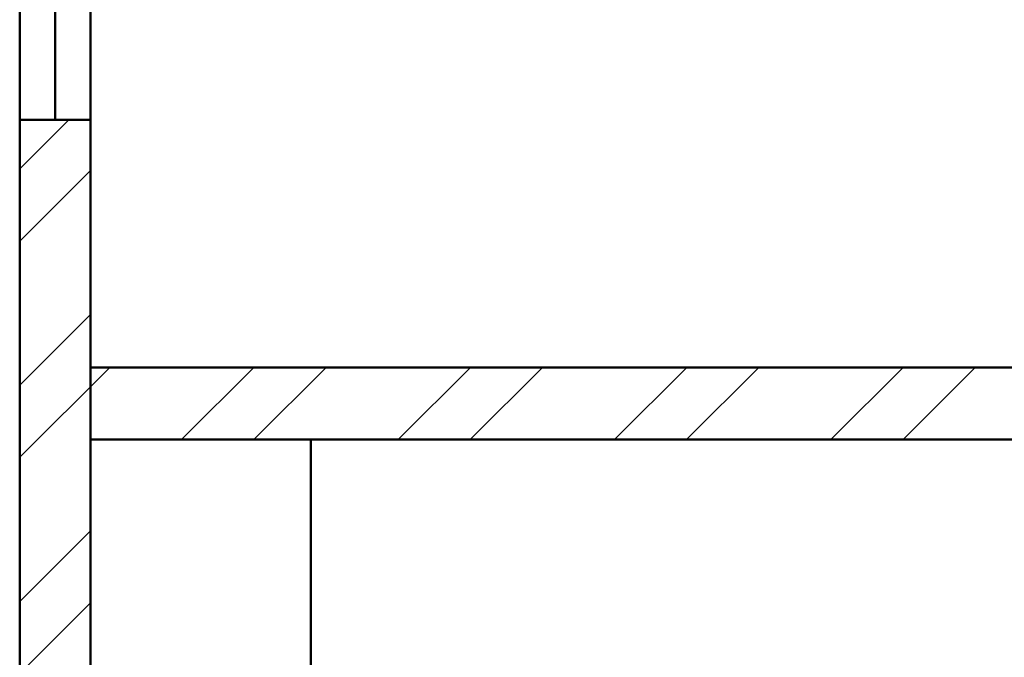
# Model space of a CAD drawing. Units: inches. Extents: x 1901 to 2863, y 888 to 2433.
# Tile 7 of 91: x 2025 to 2086, y 1510 to 1549. Entities that reach past the tile are written whole.
import ezdxf

# ---------------------------------------------------------------- set-up
doc = ezdxf.new("R2010")
doc.units = ezdxf.units.IN
doc.layers.add('A-WALL', color=7, linetype='Continuous', lineweight=50)
doc.layers.add('A-WALL-PATT', color=8, linetype='Continuous', lineweight=13)

msp = doc.modelspace()

# ---------------------------------------------------------------- hatches: boundary and pattern name
at = {"layer": 'A-WALL-PATT'}
h = msp.add_hatch(dxfattribs=at)
h.set_pattern_fill('ANSI32', color=256)
h.paths.add_polyline_path([(2182.933, 1716.634), (2024.926, 1716.634), (2024.926, 1681.702), (2029.326, 1681.702), (2029.326, 1712.134), (2154.326, 1712.134), (2154.326, 1580.134), (2148.524, 1580.134), (2148.524, 1577.884), (2148.524, 1575.634), (2194.93, 1575.634), (2194.93, 1580.134), (2158.826, 1580.134), (2158.826, 1712.134), (2182.933, 1712.134)])
h.paths.add_polyline_path([(2301.069, 1716.634), (2242.933, 1716.634), (2242.933, 1712.134), (2283.826, 1712.134), (2283.826, 1685.535), (2288.326, 1685.535), (2288.326, 1712.134), (2301.069, 1712.134)])
h.paths.add_polyline_path([(2288.326, 1600.411), (2286.076, 1600.411), (2283.826, 1600.411), (2283.826, 1580.134), (2270.601, 1580.134), (2270.601, 1575.634), (2288.326, 1575.634)])
h.paths.add_polyline_path([(2295.926, 1953.634), (2271.447, 1953.634), (2271.447, 1949.134), (2291.426, 1949.134), (2291.426, 1941.244), (2295.926, 1941.244)])
h.paths.add_polyline_path([(2098.376, 1244.134), (2082.326, 1244.134), (2082.326, 1302.134), (2086.523, 1302.134), (2086.523, 1306.634), (2067.456, 1306.634), (2067.456, 1302.134), (2077.826, 1302.134), (2077.826, 1239.634), (2098.376, 1239.634), (2098.376, 1241.884)])
h.paths.add_polyline_path([(2217.308, 1306.634), (2158.826, 1306.634), (2158.826, 1451.634), (2162.716, 1451.634), (2162.716, 1453.884), (2162.716, 1456.134), (2154.326, 1456.134), (2154.326, 1443.134), (2151.91, 1443.134), (2151.91, 1438.634), (2154.326, 1438.634), (2154.326, 1306.634), (2109.307, 1306.634), (2109.307, 1304.384), (2109.307, 1302.134), (2154.326, 1302.134), (2154.326, 1244.134), (2122.376, 1244.134), (2122.376, 1239.634), (2154.326, 1239.634), (2154.326, 1223.634), (2163.326, 1223.634), (2181.008, 1223.634), (2181.008, 1225.884), (2181.008, 1228.134), (2163.326, 1228.134), (2163.326, 1258.222), (2158.826, 1258.222), (2158.826, 1302.134), (2217.308, 1302.134)])
h.paths.add_polyline_path([(2259.991, 1306.634), (2238.299, 1306.634), (2238.299, 1304.384), (2238.299, 1302.134), (2242.826, 1302.134), (2242.826, 1228.134), (2205.008, 1228.134), (2205.008, 1223.634), (2247.326, 1223.634), (2247.326, 1302.134), (2259.991, 1302.134), (2259.991, 1304.384)])
h.paths.add_polyline_path([(2343.426, 1361.697), (2338.926, 1361.697), (2338.926, 1306.634), (2322.38, 1306.634), (2322.38, 1302.134), (2343.426, 1302.134)])
h.paths.add_polyline_path([(2343.426, 1470.397), (2338.926, 1470.397), (2338.926, 1456.134), (2193.726, 1456.134), (2193.726, 1453.884), (2193.726, 1451.634), (2338.926, 1451.634), (2338.926, 1421.697), (2343.426, 1421.697)])
h.paths.add_polyline_path([(2343.426, 1545.507), (2338.926, 1545.507), (2338.926, 1530.397), (2343.426, 1530.397)])
h.paths.add_polyline_path([(2029.326, 1466.83), (2024.926, 1466.83), (2024.926, 1409.825), (2029.326, 1409.825)])
h.paths.add_polyline_path([(2122.843, 1440.884), (2122.843, 1443.134), (2121.826, 1443.134), (2121.826, 1498.183), (2119.576, 1498.183), (2117.326, 1498.183), (2117.326, 1443.134), (2029.326, 1443.134), (2029.326, 1438.634), (2122.843, 1438.634)])
h.paths.add_polyline_path([(2029.326, 1543.053), (2024.926, 1543.053), (2024.926, 1502.83), (2029.326, 1502.83)])
h.paths.add_polyline_path([(2029.326, 1621.702), (2024.926, 1621.702), (2024.926, 1567.053), (2027.126, 1567.053), (2029.326, 1567.053), (2029.326, 1575.634), (2109.326, 1575.634), (2109.326, 1554.715), (2113.826, 1554.715), (2113.826, 1575.634), (2115.805, 1575.634), (2115.805, 1577.884), (2115.805, 1580.134), (2029.326, 1580.134)])
h.paths.add_polyline_path([(2121.826, 1527.634), (2117.326, 1527.634), (2113.826, 1527.634), (2113.826, 1533.011), (2111.576, 1533.011), (2109.326, 1533.011), (2109.326, 1527.634), (2029.326, 1527.634), (2029.326, 1523.134), (2117.326, 1523.134), (2117.326, 1519.43), (2121.826, 1519.43)])
h.paths.add_polyline_path([(2029.326, 1349.825), (2024.926, 1349.825), (2024.926, 1302.134), (2036.277, 1302.134), (2036.277, 1306.634), (2029.326, 1306.634)])

# ---------------------------------------------------------------- linework, layer by layer
at = {"layer": 'A-WALL'}
for p, q in [((2024.926, 1716.634), (2024.926, 1302.134)), ((2029.326, 1575.634), (2029.326, 1306.634)), ((2027.126, 1567.053), (2027.126, 1543.053)), ((2027.126, 1543.053), (2024.926, 1543.053)), ((2024.926, 1543.053), (2029.326, 1543.053)), ((2109.326, 1527.634), (2029.326, 1527.634)), ((2117.326, 1523.134), (2029.326, 1523.134)), ((2043.059, 1456.597), (2043.059, 1523.134))]:
    msp.add_line(p, q, dxfattribs=at)

doc.saveas('drawing.dxf')
